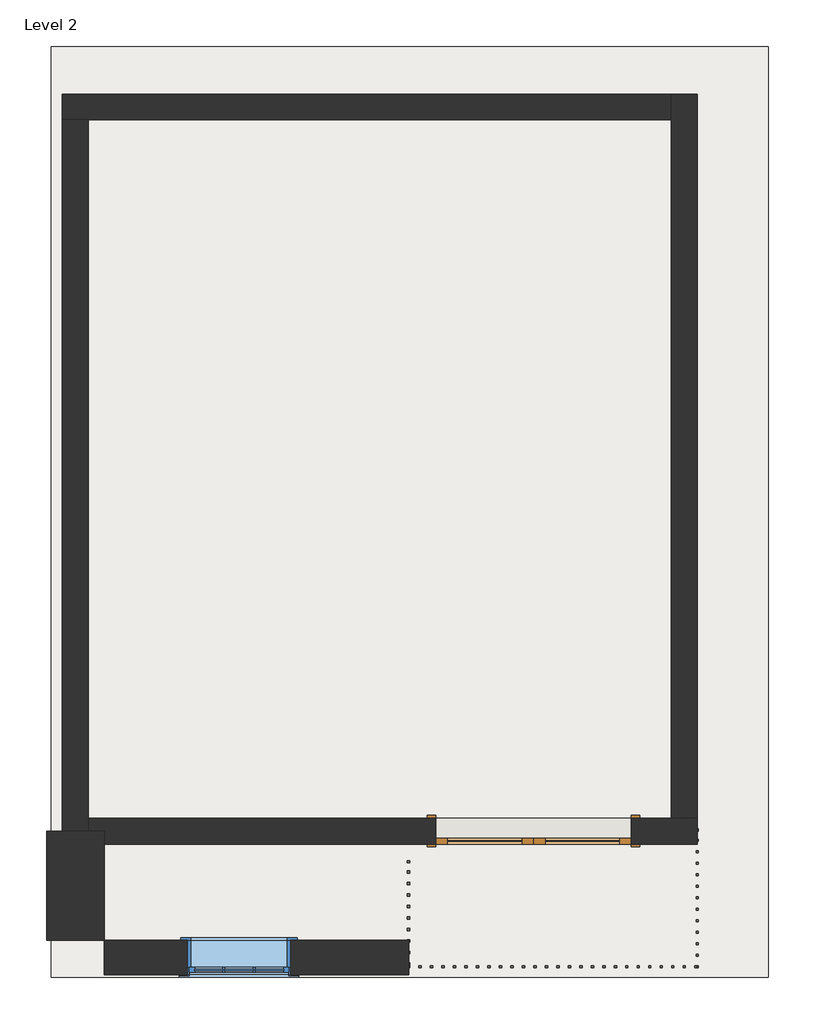
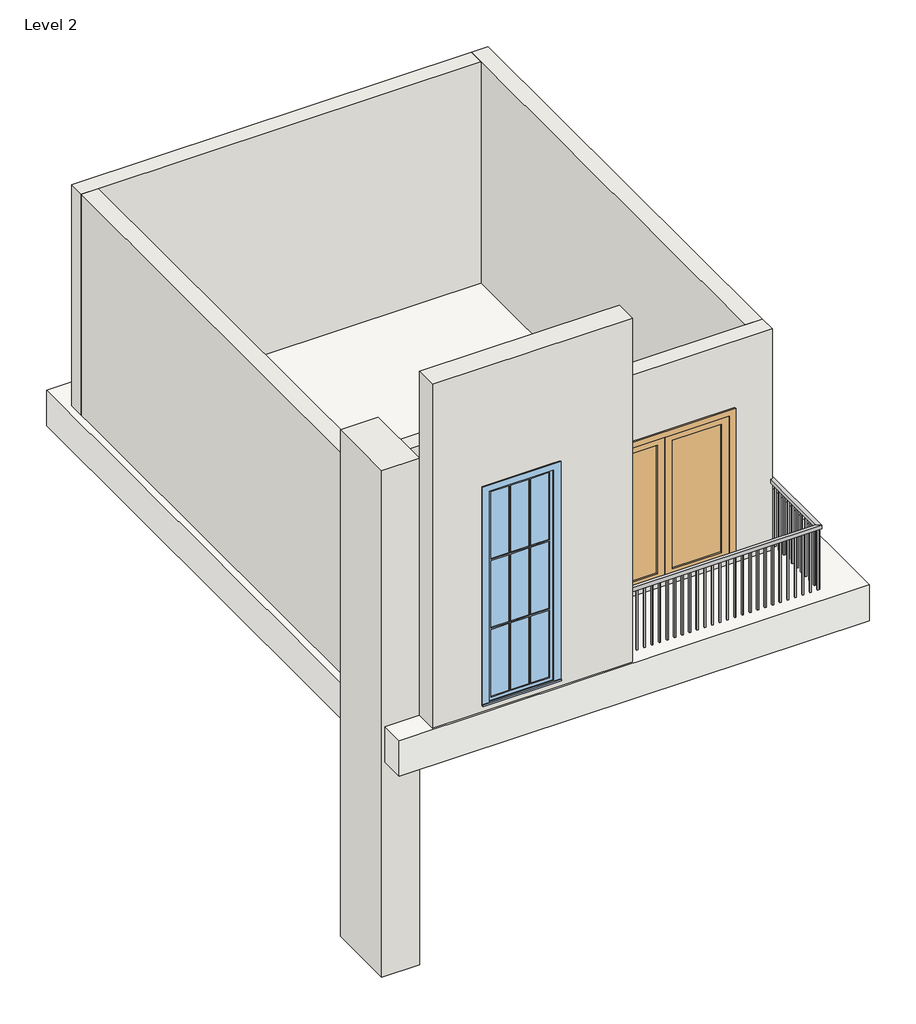
# One storey: 6 walls, 1 door, 1 railing, 1 roof, 1 window.
"""IFC4 building model written with IfcOpenShell, lengths in millimetres."""

from ifc_helpers import new_model, si_unit, frame, origin, place, context, project, spatial, polyline, outline, extrude, faceted_brep, transform, mapped, element, save
from components import door_423d55ee, window_19f256ab

model = new_model("IFC4")

# Units and contexts
model_context = context("Model", 3, world=origin())
ifc_project = project(units=[si_unit("LENGTHUNIT", "METRE", prefix="MILLI")], contexts=[model_context])

# Site, building, storey
site = spatial("IfcSite", under=ifc_project)
building = spatial("IfcBuilding", under=site)
storey = spatial("IfcBuildingStorey", under=building, Name="Level 2", Elevation=3048.0)

# Door
placement = place(None, origin())
door_shape = door_423d55ee(model_context)
element("IfcDoor", 1, ObjectType="Door-Double-Glass : 68\" x 80\"", at=placement, inside=storey, context=model_context, shape_type="MappedRepresentation", body=[
    mapped(door_shape, transform((-9039.9306534, 4280.4110237, 3657.6), x_axis=(-1.0, 0.0, 0.0), y_axis=(0.0, -1.0, 0.0), z_axis=(0.0, 0.0, 1.0))),
])

# Railing
element("IfcRailing", 2, ObjectType="Handrail - Rectangular", at=placement, inside=storey, context=model_context, shape_type="SolidModel", body=[
    faceted_brep([(-10119.4306534, 4017.6797737, 4572.0), (-10119.4306534, 4017.6797737, 4521.2), (-10170.2306534, 4017.6797737, 4521.2), (-10170.2306534, 4017.6797737, 4572.0), (-10119.4306534, 3103.2797737, 4572.0), (-10119.4306534, 3103.2797737, 4521.2), (-10170.2306534, 3052.4797737, 4521.2), (-10170.2306534, 3052.4797737, 4572.0), (-7617.5306534, 3103.2797737, 4572.0), (-7617.5306534, 3103.2797737, 4521.2), (-7566.7306534, 3052.4797737, 4521.2), (-7566.7306534, 3052.4797737, 4572.0), (-7617.5306534, 4297.0797737, 4572.0), (-7566.7306534, 4297.0797737, 4572.0), (-7566.7306534, 4297.0797737, 4521.2), (-7617.5306534, 4297.0797737, 4521.2)], [[[0, 1, 2, 3]], [[1, 0, 4, 5]], [[2, 1, 5, 6]], [[3, 2, 6, 7]], [[0, 3, 7, 4]], [[5, 4, 8, 9]], [[6, 5, 9, 10]], [[7, 6, 10, 11]], [[4, 7, 11, 8]], [[12, 13, 14, 15]], [[9, 8, 12, 15]], [[10, 9, 15, 14]], [[11, 10, 14, 13]], [[8, 11, 13, 12]]]),
    extrude(outline(polyline([(-7582.6056534, 4185.9547737), (-7601.6556534, 4185.9547737), (-7601.6556534, 4205.0047737), (-7582.6056534, 4205.0047737), (-7582.6056534, 4185.9547737)])), frame((0.0, 0.0, 3657.6), z_axis=(0.0, 0.0, 1.0), x_axis=(1.0, 0.0, 0.0)), (0.0, 0.0, 1.0), 863.6),
    extrude(outline(polyline([(-7582.6056534, 4084.3547737), (-7601.6556534, 4084.3547737), (-7601.6556534, 4103.4047737), (-7582.6056534, 4103.4047737), (-7582.6056534, 4084.3547737)])), frame((0.0, 0.0, 3657.6), z_axis=(0.0, 0.0, 1.0), x_axis=(1.0, 0.0, 0.0)), (0.0, 0.0, 1.0), 863.6),
    extrude(outline(polyline([(-7582.6056534, 3982.7547737), (-7601.6556534, 3982.7547737), (-7601.6556534, 4001.8047737), (-7582.6056534, 4001.8047737), (-7582.6056534, 3982.7547737)])), frame((0.0, 0.0, 3657.6), z_axis=(0.0, 0.0, 1.0), x_axis=(1.0, 0.0, 0.0)), (0.0, 0.0, 1.0), 863.6),
    extrude(outline(polyline([(-7582.6056534, 3881.1547737), (-7601.6556534, 3881.1547737), (-7601.6556534, 3900.2047737), (-7582.6056534, 3900.2047737), (-7582.6056534, 3881.1547737)])), frame((0.0, 0.0, 3657.6), z_axis=(0.0, 0.0, 1.0), x_axis=(1.0, 0.0, 0.0)), (0.0, 0.0, 1.0), 863.6),
    extrude(outline(polyline([(-7582.6056534, 3779.5547737), (-7601.6556534, 3779.5547737), (-7601.6556534, 3798.6047737), (-7582.6056534, 3798.6047737), (-7582.6056534, 3779.5547737)])), frame((0.0, 0.0, 3657.6), z_axis=(0.0, 0.0, 1.0), x_axis=(1.0, 0.0, 0.0)), (0.0, 0.0, 1.0), 863.6),
    extrude(outline(polyline([(-7582.6056534, 3677.9547737), (-7601.6556534, 3677.9547737), (-7601.6556534, 3697.0047737), (-7582.6056534, 3697.0047737), (-7582.6056534, 3677.9547737)])), frame((0.0, 0.0, 3657.6), z_axis=(0.0, 0.0, 1.0), x_axis=(1.0, 0.0, 0.0)), (0.0, 0.0, 1.0), 863.6),
    extrude(outline(polyline([(-7582.6056534, 3576.3547737), (-7601.6556534, 3576.3547737), (-7601.6556534, 3595.4047737), (-7582.6056534, 3595.4047737), (-7582.6056534, 3576.3547737)])), frame((0.0, 0.0, 3657.6), z_axis=(0.0, 0.0, 1.0), x_axis=(1.0, 0.0, 0.0)), (0.0, 0.0, 1.0), 863.6),
    extrude(outline(polyline([(-7582.6056534, 3474.7547737), (-7601.6556534, 3474.7547737), (-7601.6556534, 3493.8047737), (-7582.6056534, 3493.8047737), (-7582.6056534, 3474.7547737)])), frame((0.0, 0.0, 3657.6), z_axis=(0.0, 0.0, 1.0), x_axis=(1.0, 0.0, 0.0)), (0.0, 0.0, 1.0), 863.6),
    extrude(outline(polyline([(-7582.6056534, 3373.1547737), (-7601.6556534, 3373.1547737), (-7601.6556534, 3392.2047737), (-7582.6056534, 3392.2047737), (-7582.6056534, 3373.1547737)])), frame((0.0, 0.0, 3657.6), z_axis=(0.0, 0.0, 1.0), x_axis=(1.0, 0.0, 0.0)), (0.0, 0.0, 1.0), 863.6),
    extrude(outline(polyline([(-7582.6056534, 3271.5547737), (-7601.6556534, 3271.5547737), (-7601.6556534, 3290.6047737), (-7582.6056534, 3290.6047737), (-7582.6056534, 3271.5547737)])), frame((0.0, 0.0, 3657.6), z_axis=(0.0, 0.0, 1.0), x_axis=(1.0, 0.0, 0.0)), (0.0, 0.0, 1.0), 863.6),
    extrude(outline(polyline([(-7582.6056534, 3169.9547737), (-7601.6556534, 3169.9547737), (-7601.6556534, 3189.0047737), (-7582.6056534, 3189.0047737), (-7582.6056534, 3169.9547737)])), frame((0.0, 0.0, 3657.6), z_axis=(0.0, 0.0, 1.0), x_axis=(1.0, 0.0, 0.0)), (0.0, 0.0, 1.0), 863.6),
    extrude(outline(polyline([(-7614.3556534, 3068.3547737), (-7614.3556534, 3087.4047737), (-7595.3056534, 3087.4047737), (-7595.3056534, 3068.3547737), (-7614.3556534, 3068.3547737)])), frame((0.0, 0.0, 3657.6), z_axis=(0.0, 0.0, 1.0), x_axis=(1.0, 0.0, 0.0)), (0.0, 0.0, 1.0), 863.6),
    extrude(outline(polyline([(-7715.9556534, 3068.3547737), (-7715.9556534, 3087.4047737), (-7696.9056534, 3087.4047737), (-7696.9056534, 3068.3547737), (-7715.9556534, 3068.3547737)])), frame((0.0, 0.0, 3657.6), z_axis=(0.0, 0.0, 1.0), x_axis=(1.0, 0.0, 0.0)), (0.0, 0.0, 1.0), 863.6),
    extrude(outline(polyline([(-7817.5556534, 3068.3547737), (-7817.5556534, 3087.4047737), (-7798.5056534, 3087.4047737), (-7798.5056534, 3068.3547737), (-7817.5556534, 3068.3547737)])), frame((0.0, 0.0, 3657.6), z_axis=(0.0, 0.0, 1.0), x_axis=(1.0, 0.0, 0.0)), (0.0, 0.0, 1.0), 863.6),
    extrude(outline(polyline([(-7919.1556534, 3068.3547737), (-7919.1556534, 3087.4047737), (-7900.1056534, 3087.4047737), (-7900.1056534, 3068.3547737), (-7919.1556534, 3068.3547737)])), frame((0.0, 0.0, 3657.6), z_axis=(0.0, 0.0, 1.0), x_axis=(1.0, 0.0, 0.0)), (0.0, 0.0, 1.0), 863.6),
    extrude(outline(polyline([(-8020.7556534, 3068.3547737), (-8020.7556534, 3087.4047737), (-8001.7056534, 3087.4047737), (-8001.7056534, 3068.3547737), (-8020.7556534, 3068.3547737)])), frame((0.0, 0.0, 3657.6), z_axis=(0.0, 0.0, 1.0), x_axis=(1.0, 0.0, 0.0)), (0.0, 0.0, 1.0), 863.6),
    extrude(outline(polyline([(-8122.3556534, 3068.3547737), (-8122.3556534, 3087.4047737), (-8103.3056534, 3087.4047737), (-8103.3056534, 3068.3547737), (-8122.3556534, 3068.3547737)])), frame((0.0, 0.0, 3657.6), z_axis=(0.0, 0.0, 1.0), x_axis=(1.0, 0.0, 0.0)), (0.0, 0.0, 1.0), 863.6),
    extrude(outline(polyline([(-8223.9556534, 3068.3547737), (-8223.9556534, 3087.4047737), (-8204.9056534, 3087.4047737), (-8204.9056534, 3068.3547737), (-8223.9556534, 3068.3547737)])), frame((0.0, 0.0, 3657.6), z_axis=(0.0, 0.0, 1.0), x_axis=(1.0, 0.0, 0.0)), (0.0, 0.0, 1.0), 863.6),
    extrude(outline(polyline([(-8325.5556534, 3068.3547737), (-8325.5556534, 3087.4047737), (-8306.5056534, 3087.4047737), (-8306.5056534, 3068.3547737), (-8325.5556534, 3068.3547737)])), frame((0.0, 0.0, 3657.6), z_axis=(0.0, 0.0, 1.0), x_axis=(1.0, 0.0, 0.0)), (0.0, 0.0, 1.0), 863.6),
    extrude(outline(polyline([(-8427.1556534, 3068.3547737), (-8427.1556534, 3087.4047737), (-8408.1056534, 3087.4047737), (-8408.1056534, 3068.3547737), (-8427.1556534, 3068.3547737)])), frame((0.0, 0.0, 3657.6), z_axis=(0.0, 0.0, 1.0), x_axis=(1.0, 0.0, 0.0)), (0.0, 0.0, 1.0), 863.6),
    extrude(outline(polyline([(-8528.7556534, 3068.3547737), (-8528.7556534, 3087.4047737), (-8509.7056534, 3087.4047737), (-8509.7056534, 3068.3547737), (-8528.7556534, 3068.3547737)])), frame((0.0, 0.0, 3657.6), z_axis=(0.0, 0.0, 1.0), x_axis=(1.0, 0.0, 0.0)), (0.0, 0.0, 1.0), 863.6),
    extrude(outline(polyline([(-8630.3556534, 3068.3547737), (-8630.3556534, 3087.4047737), (-8611.3056534, 3087.4047737), (-8611.3056534, 3068.3547737), (-8630.3556534, 3068.3547737)])), frame((0.0, 0.0, 3657.6), z_axis=(0.0, 0.0, 1.0), x_axis=(1.0, 0.0, 0.0)), (0.0, 0.0, 1.0), 863.6),
    extrude(outline(polyline([(-8731.9556534, 3068.3547737), (-8731.9556534, 3087.4047737), (-8712.9056534, 3087.4047737), (-8712.9056534, 3068.3547737), (-8731.9556534, 3068.3547737)])), frame((0.0, 0.0, 3657.6), z_axis=(0.0, 0.0, 1.0), x_axis=(1.0, 0.0, 0.0)), (0.0, 0.0, 1.0), 863.6),
    extrude(outline(polyline([(-8833.5556534, 3068.3547737), (-8833.5556534, 3087.4047737), (-8814.5056534, 3087.4047737), (-8814.5056534, 3068.3547737), (-8833.5556534, 3068.3547737)])), frame((0.0, 0.0, 3657.6), z_axis=(0.0, 0.0, 1.0), x_axis=(1.0, 0.0, 0.0)), (0.0, 0.0, 1.0), 863.6),
    extrude(outline(polyline([(-8935.1556534, 3068.3547737), (-8935.1556534, 3087.4047737), (-8916.1056534, 3087.4047737), (-8916.1056534, 3068.3547737), (-8935.1556534, 3068.3547737)])), frame((0.0, 0.0, 3657.6), z_axis=(0.0, 0.0, 1.0), x_axis=(1.0, 0.0, 0.0)), (0.0, 0.0, 1.0), 863.6),
    extrude(outline(polyline([(-9036.7556534, 3068.3547737), (-9036.7556534, 3087.4047737), (-9017.7056534, 3087.4047737), (-9017.7056534, 3068.3547737), (-9036.7556534, 3068.3547737)])), frame((0.0, 0.0, 3657.6), z_axis=(0.0, 0.0, 1.0), x_axis=(1.0, 0.0, 0.0)), (0.0, 0.0, 1.0), 863.6),
    extrude(outline(polyline([(-9138.3556534, 3068.3547737), (-9138.3556534, 3087.4047737), (-9119.3056534, 3087.4047737), (-9119.3056534, 3068.3547737), (-9138.3556534, 3068.3547737)])), frame((0.0, 0.0, 3657.6), z_axis=(0.0, 0.0, 1.0), x_axis=(1.0, 0.0, 0.0)), (0.0, 0.0, 1.0), 863.6),
    extrude(outline(polyline([(-9239.9556534, 3068.3547737), (-9239.9556534, 3087.4047737), (-9220.9056534, 3087.4047737), (-9220.9056534, 3068.3547737), (-9239.9556534, 3068.3547737)])), frame((0.0, 0.0, 3657.6), z_axis=(0.0, 0.0, 1.0), x_axis=(1.0, 0.0, 0.0)), (0.0, 0.0, 1.0), 863.6),
    extrude(outline(polyline([(-9341.5556534, 3068.3547737), (-9341.5556534, 3087.4047737), (-9322.5056534, 3087.4047737), (-9322.5056534, 3068.3547737), (-9341.5556534, 3068.3547737)])), frame((0.0, 0.0, 3657.6), z_axis=(0.0, 0.0, 1.0), x_axis=(1.0, 0.0, 0.0)), (0.0, 0.0, 1.0), 863.6),
    extrude(outline(polyline([(-9443.1556534, 3068.3547737), (-9443.1556534, 3087.4047737), (-9424.1056534, 3087.4047737), (-9424.1056534, 3068.3547737), (-9443.1556534, 3068.3547737)])), frame((0.0, 0.0, 3657.6), z_axis=(0.0, 0.0, 1.0), x_axis=(1.0, 0.0, 0.0)), (0.0, 0.0, 1.0), 863.6),
    extrude(outline(polyline([(-9544.7556534, 3068.3547737), (-9544.7556534, 3087.4047737), (-9525.7056534, 3087.4047737), (-9525.7056534, 3068.3547737), (-9544.7556534, 3068.3547737)])), frame((0.0, 0.0, 3657.6), z_axis=(0.0, 0.0, 1.0), x_axis=(1.0, 0.0, 0.0)), (0.0, 0.0, 1.0), 863.6),
    extrude(outline(polyline([(-9646.3556534, 3068.3547737), (-9646.3556534, 3087.4047737), (-9627.3056534, 3087.4047737), (-9627.3056534, 3068.3547737), (-9646.3556534, 3068.3547737)])), frame((0.0, 0.0, 3657.6), z_axis=(0.0, 0.0, 1.0), x_axis=(1.0, 0.0, 0.0)), (0.0, 0.0, 1.0), 863.6),
    extrude(outline(polyline([(-9747.9556534, 3068.3547737), (-9747.9556534, 3087.4047737), (-9728.9056534, 3087.4047737), (-9728.9056534, 3068.3547737), (-9747.9556534, 3068.3547737)])), frame((0.0, 0.0, 3657.6), z_axis=(0.0, 0.0, 1.0), x_axis=(1.0, 0.0, 0.0)), (0.0, 0.0, 1.0), 863.6),
    extrude(outline(polyline([(-9849.5556534, 3068.3547737), (-9849.5556534, 3087.4047737), (-9830.5056534, 3087.4047737), (-9830.5056534, 3068.3547737), (-9849.5556534, 3068.3547737)])), frame((0.0, 0.0, 3657.6), z_axis=(0.0, 0.0, 1.0), x_axis=(1.0, 0.0, 0.0)), (0.0, 0.0, 1.0), 863.6),
    extrude(outline(polyline([(-9951.1556534, 3068.3547737), (-9951.1556534, 3087.4047737), (-9932.1056534, 3087.4047737), (-9932.1056534, 3068.3547737), (-9951.1556534, 3068.3547737)])), frame((0.0, 0.0, 3657.6), z_axis=(0.0, 0.0, 1.0), x_axis=(1.0, 0.0, 0.0)), (0.0, 0.0, 1.0), 863.6),
    extrude(outline(polyline([(-10052.7556534, 3068.3547737), (-10052.7556534, 3087.4047737), (-10033.7056534, 3087.4047737), (-10033.7056534, 3068.3547737), (-10052.7556534, 3068.3547737)])), frame((0.0, 0.0, 3657.6), z_axis=(0.0, 0.0, 1.0), x_axis=(1.0, 0.0, 0.0)), (0.0, 0.0, 1.0), 863.6),
    extrude(outline(polyline([(-10154.3556534, 3112.8047737), (-10135.3056534, 3112.8047737), (-10135.3056534, 3093.7547737), (-10154.3556534, 3093.7547737), (-10154.3556534, 3112.8047737)])), frame((0.0, 0.0, 3657.6), z_axis=(0.0, 0.0, 1.0), x_axis=(1.0, 0.0, 0.0)), (0.0, 0.0, 1.0), 863.6),
    extrude(outline(polyline([(-10154.3556534, 3214.4047737), (-10135.3056534, 3214.4047737), (-10135.3056534, 3195.3547737), (-10154.3556534, 3195.3547737), (-10154.3556534, 3214.4047737)])), frame((0.0, 0.0, 3657.6), z_axis=(0.0, 0.0, 1.0), x_axis=(1.0, 0.0, 0.0)), (0.0, 0.0, 1.0), 863.6),
    extrude(outline(polyline([(-10154.3556534, 3316.0047737), (-10135.3056534, 3316.0047737), (-10135.3056534, 3296.9547737), (-10154.3556534, 3296.9547737), (-10154.3556534, 3316.0047737)])), frame((0.0, 0.0, 3657.6), z_axis=(0.0, 0.0, 1.0), x_axis=(1.0, 0.0, 0.0)), (0.0, 0.0, 1.0), 863.6),
    extrude(outline(polyline([(-10154.3556534, 3417.6047737), (-10135.3056534, 3417.6047737), (-10135.3056534, 3398.5547737), (-10154.3556534, 3398.5547737), (-10154.3556534, 3417.6047737)])), frame((0.0, 0.0, 3657.6), z_axis=(0.0, 0.0, 1.0), x_axis=(1.0, 0.0, 0.0)), (0.0, 0.0, 1.0), 863.6),
    extrude(outline(polyline([(-10154.3556534, 3519.2047737), (-10135.3056534, 3519.2047737), (-10135.3056534, 3500.1547737), (-10154.3556534, 3500.1547737), (-10154.3556534, 3519.2047737)])), frame((0.0, 0.0, 3657.6), z_axis=(0.0, 0.0, 1.0), x_axis=(1.0, 0.0, 0.0)), (0.0, 0.0, 1.0), 863.6),
    extrude(outline(polyline([(-10154.3556534, 3620.8047737), (-10135.3056534, 3620.8047737), (-10135.3056534, 3601.7547737), (-10154.3556534, 3601.7547737), (-10154.3556534, 3620.8047737)])), frame((0.0, 0.0, 3657.6), z_axis=(0.0, 0.0, 1.0), x_axis=(1.0, 0.0, 0.0)), (0.0, 0.0, 1.0), 863.6),
    extrude(outline(polyline([(-10154.3556534, 3722.4047737), (-10135.3056534, 3722.4047737), (-10135.3056534, 3703.3547737), (-10154.3556534, 3703.3547737), (-10154.3556534, 3722.4047737)])), frame((0.0, 0.0, 3657.6), z_axis=(0.0, 0.0, 1.0), x_axis=(1.0, 0.0, 0.0)), (0.0, 0.0, 1.0), 863.6),
    extrude(outline(polyline([(-10154.3556534, 3824.0047737), (-10135.3056534, 3824.0047737), (-10135.3056534, 3804.9547737), (-10154.3556534, 3804.9547737), (-10154.3556534, 3824.0047737)])), frame((0.0, 0.0, 3657.6), z_axis=(0.0, 0.0, 1.0), x_axis=(1.0, 0.0, 0.0)), (0.0, 0.0, 1.0), 863.6),
    extrude(outline(polyline([(-10154.3556534, 3925.6047737), (-10135.3056534, 3925.6047737), (-10135.3056534, 3906.5547737), (-10154.3556534, 3906.5547737), (-10154.3556534, 3925.6047737)])), frame((0.0, 0.0, 3657.6), z_axis=(0.0, 0.0, 1.0), x_axis=(1.0, 0.0, 0.0)), (0.0, 0.0, 1.0), 863.6),
    extrude(outline(polyline([(-7601.6556534, 3068.3547737), (-7601.6556534, 3087.4047737), (-7582.6056534, 3087.4047737), (-7582.6056534, 3068.3547737), (-7601.6556534, 3068.3547737)])), frame((0.0, 0.0, 3657.6), z_axis=(0.0, 0.0, 1.0), x_axis=(1.0, 0.0, 0.0)), (0.0, 0.0, 1.0), 863.6),
    extrude(outline(polyline([(-10154.3556534, 3087.4047737), (-10135.3056534, 3087.4047737), (-10135.3056534, 3068.3547737), (-10154.3556534, 3068.3547737), (-10154.3556534, 3087.4047737)])), frame((0.0, 0.0, 3657.6), z_axis=(0.0, 0.0, 1.0), x_axis=(1.0, 0.0, 0.0)), (0.0, 0.0, 1.0), 863.6),
    extrude(outline(polyline([(-7582.6056534, 4278.0297737), (-7601.6556534, 4278.0297737), (-7601.6556534, 4297.0797737), (-7582.6056534, 4297.0797737), (-7582.6056534, 4278.0297737)])), frame((0.0, 0.0, 3657.6), z_axis=(0.0, 0.0, 1.0), x_axis=(1.0, 0.0, 0.0)), (0.0, 0.0, 1.0), 863.6),
    extrude(outline(polyline([(-10154.3556534, 4017.6797737), (-10135.3056534, 4017.6797737), (-10135.3056534, 3998.6297737), (-10154.3556534, 3998.6297737), (-10154.3556534, 4017.6797737)])), frame((0.0, 0.0, 3657.6), z_axis=(0.0, 0.0, 1.0), x_axis=(1.0, 0.0, 0.0)), (0.0, 0.0, 1.0), 863.6),
])

# Roof
element("IfcRoof", 3, ObjectType="Generic - 18\"", at=placement, inside=storey, context=model_context, shape_type="SweptSolid", body=[
    extrude(outline(polyline([(-13301.4465329, 11213.7598519), (-6964.1465329, 11213.7598519), (-6964.1465329, 2984.1598519), (-13301.4465329, 2984.1598519), (-13301.4465329, 11213.7598519)])), frame((0.0, 0.0, 3048.0), z_axis=(0.0, 0.0, 1.0), x_axis=(1.0, 0.0, 0.0)), (0.0, 0.0, 1.0), 508.0),
])

# Walls
element("IfcWall", 4, ObjectType="Generic - 12\"", at=placement, inside=storey, context=model_context, shape_type="Brep", body=[
    faceted_brep([(-10144.8306534, 3314.3598519, 3048.0), (-12837.2306534, 3314.3598519, 3048.0), (-12837.2306534, 3314.3598519, 8451.8321088), (-10449.6306534, 3314.3598519, 8451.8321088), (-10144.8306534, 3314.3598519, 8451.8321088), (-12100.6306534, 3314.3598519, 6693.08663), (-12100.6306534, 3314.3598519, 3645.08663), (-11186.2306534, 3314.3598519, 3645.08663), (-11186.2306534, 3314.3598519, 6693.08663), (-10144.8306534, 3009.5598519, 3048.0), (-10144.8306534, 3009.5598519, 8451.8321088), (-12837.2306534, 3009.5598519, 8451.8321088), (-12837.2306534, 3009.5598519, 3048.0), (-12100.6306534, 3009.5598519, 6693.08663), (-11186.2306534, 3009.5598519, 6693.08663), (-11186.2306534, 3009.5598519, 3645.08663), (-12100.6306534, 3009.5598519, 3645.08663)], [[[0, 1, 2, 3, 4], [5, 6, 7, 8]], [[9, 10, 11, 12], [13, 14, 15, 16]], [[6, 5, 13, 16]], [[7, 6, 16, 15]], [[8, 7, 15, 14]], [[5, 8, 14, 13]], [[1, 0, 9, 12]], [[4, 3, 2, 11, 10]], [[2, 1, 12, 11]], [[0, 4, 10, 9]]]),
])
element("IfcWall", 5, ObjectType="Generic - 12\" Masonry", at=placement, inside=storey, context=model_context, shape_type="Brep", body=[
    faceted_brep([(-13345.2306534, 4278.0297737, 7213.6), (-13345.2306534, 4278.0297737, 0.0), (-13345.2306534, 3314.3598519, 0.0), (-13345.2306534, 3314.3598519, 6705.6), (-13345.2306534, 3314.3598519, 7213.6), (-12837.2306534, 4278.0297737, 0.0), (-12837.2306534, 4278.0297737, 3048.0), (-12837.2306534, 4278.0297737, 6705.6), (-12837.2306534, 4278.0297737, 7213.6), (-12837.2306534, 3314.3598519, 7213.6), (-12837.2306534, 3314.3598519, 6705.6), (-12837.2306534, 3314.3598519, 0.0), (-12837.2306534, 4163.7297737, 0.0), (-13205.5306534, 4278.0297737, 0.0), (-12976.9306534, 4278.0297737, 0.0)], [[[0, 1, 2, 3, 4]], [[5, 6, 7, 8, 9, 10, 11, 12]], [[2, 1, 13, 14, 5, 12, 11]], [[0, 4, 9, 8]], [[0, 8, 7, 6, 5, 14, 13, 1]], [[4, 3, 2, 11, 10, 9]]]),
])
element("IfcWall", 6, ObjectType="Generic - 9\"", at=placement, inside=storey, context=model_context, shape_type="Brep", body=[
    faceted_brep([(-13205.5306534, 10564.5297737, 6705.6), (-13205.5306534, 10564.5297737, 3048.0), (-12976.9306534, 10564.5297737, 3048.0), (-7820.7306534, 10564.5297737, 3048.0), (-7820.7306534, 10564.5297737, 6705.6), (-12976.9306534, 10564.5297737, 6705.6), (-13205.5306534, 10793.1297737, 3048.0), (-13205.5306534, 10793.1297737, 6705.6), (-7820.7306534, 10793.1297737, 6705.6), (-7820.7306534, 10793.1297737, 3048.0)], [[[0, 1, 2, 3, 4, 5]], [[6, 7, 8, 9]], [[3, 2, 1, 6, 9]], [[0, 5, 4, 8, 7]], [[0, 7, 6, 1]], [[3, 9, 8, 4]]]),
])
element("IfcWall", 7, ObjectType="Generic - 9\"", at=placement, inside=storey, context=model_context, shape_type="Brep", body=[
    faceted_brep([(-12976.9306534, 4278.0297737, 6705.6), (-12976.9306534, 4278.0297737, 3048.0), (-12976.9306534, 4392.3297737, 3048.0), (-12976.9306534, 10564.5297737, 3048.0), (-12976.9306534, 10564.5297737, 6705.6), (-12976.9306534, 4392.3297737, 6705.6), (-13205.5306534, 4278.0297737, 3048.0), (-13205.5306534, 4278.0297737, 6705.6), (-13205.5306534, 10564.5297737, 6705.6), (-13205.5306534, 10564.5297737, 3048.0)], [[[0, 1, 2, 3, 4, 5]], [[6, 7, 8, 9]], [[3, 2, 1, 6, 9]], [[0, 5, 4, 8, 7]], [[3, 9, 8, 4]], [[0, 7, 6, 1]]]),
])
element("IfcWall", 8, ObjectType="Generic - 9\"", at=placement, inside=storey, context=model_context, shape_type="Brep", body=[
    faceted_brep([(-7592.1306534, 4392.3297737, 6705.6), (-7592.1306534, 4392.3297737, 3048.0), (-7820.7306534, 4392.3297737, 3048.0), (-12976.9306534, 4392.3297737, 3048.0), (-12976.9306534, 4392.3297737, 6705.6), (-7820.7306534, 4392.3297737, 6705.6), (-8176.3306534, 4392.3297737, 3657.6), (-8176.3306534, 4392.3297737, 5689.6), (-9903.5306534, 4392.3297737, 5689.6), (-9903.5306534, 4392.3297737, 3657.6), (-7592.1306534, 4163.7297737, 3048.0), (-7592.1306534, 4163.7297737, 6705.6), (-12837.2306534, 4163.7297737, 6705.6), (-12837.2306534, 4163.7297737, 3048.0), (-8176.3306534, 4163.7297737, 3657.6), (-9903.5306534, 4163.7297737, 3657.6), (-9903.5306534, 4163.7297737, 5689.6), (-8176.3306534, 4163.7297737, 5689.6), (-12837.2306534, 4278.0297737, 3048.0), (-12976.9306534, 4278.0297737, 3048.0), (-12976.9306534, 4278.0297737, 6705.6), (-12837.2306534, 4278.0297737, 6705.6)], [[[0, 1, 2, 3, 4, 5], [6, 7, 8, 9]], [[10, 11, 12, 13], [14, 15, 16, 17]], [[3, 2, 1, 10, 13, 18, 19]], [[0, 5, 4, 20, 21, 12, 11]], [[0, 11, 10, 1]], [[15, 14, 6, 9]], [[16, 15, 9, 8]], [[17, 16, 8, 7]], [[14, 17, 7, 6]], [[3, 19, 20, 4]], [[20, 19, 18, 21]], [[21, 18, 13, 12]]]),
])
element("IfcWall", 9, ObjectType="Generic - 9\"", at=placement, inside=storey, context=model_context, shape_type="Brep", body=[
    faceted_brep([(-7820.7306534, 10793.1297737, 6705.6), (-7820.7306534, 10793.1297737, 3048.0), (-7820.7306534, 10564.5297737, 3048.0), (-7820.7306534, 4392.3297737, 3048.0), (-7820.7306534, 4392.3297737, 6705.6), (-7820.7306534, 10564.5297737, 6705.6), (-7592.1306534, 10793.1297737, 3048.0), (-7592.1306534, 10793.1297737, 6705.6), (-7592.1306534, 4392.3297737, 6705.6), (-7592.1306534, 4392.3297737, 3048.0)], [[[0, 1, 2, 3, 4, 5]], [[6, 7, 8, 9]], [[3, 2, 1, 6, 9]], [[0, 5, 4, 8, 7]], [[3, 9, 8, 4]], [[0, 7, 6, 1]]]),
])

# Window
window_shape = window_19f256ab(model_context)
element("IfcWindow", 10, ObjectType="Casement 3x3 with Trim : 36\" x 48\"", at=placement, inside=storey, context=model_context, shape_type="MappedRepresentation", body=[
    mapped(window_shape, transform((-11643.4306534, 3161.9598519, 2730.68663), x_axis=(-1.0, 0.0, 0.0), y_axis=(0.0, -1.0, 0.0), z_axis=(0.0, 0.0, 1.0))),
])

save(model, "model.ifc")

# Revit data of these elements
# Type "Door-Double-Glass : 68\" x 80\""
#   Type Mark = "8"
#   Construction Type Id = "opn-d45"
#   Assembly Code = "C1020"
#   Analytic Construction = "Wood frame, double glass door "
#   W = 2' - 10"
#   Thickness = 0' - 2"
#   Thermal Resistance (R) = 1.8150 (h·ft²·°F)/BTU
#   Swing Angle [instance default] = 90.00°
#   Heat Transfer Coefficient (U) = 0.5510 BTU/(h·ft²·°F)
#   Height = 6' - 8"
#   Bottom Rail = 0' - 4"
#   Top Rail = 0' - 4"
#   Stiles = 0' - 4"
#   Trim Projection = 0' - 1"
#   Trim Width = 0' - 3"
#   Width = 5' - 8"
#   Define Thermal Properties by = 1
#   Glazing = Glass
#   Panel Material = Wood - Birch - Solid Stained Light Low Gloss
#   Trim Material = Paint - Sienna
#   Visual Light Transmittance = 0
#   Solar Heat Gain Coefficient = 0
#   Function = (empty or 0)
#   Wall Closure = (empty or 0)
# Type "Handrail - Rectangular"
#   Assembly Code = "C2010400"
#   built-in parameter 1008612 = 0.0416667 (stored number, unit not read)
#   built-in parameter 1008611 = 0.0416667 (stored number, unit not read)
#   built-in parameter 1008609 = 0.333333 (stored number, unit not read)
#   built-in parameter 1008604 = 0.166667 (stored number, unit not read)
#   built-in parameter 1008603 = 0.166667 (stored number, unit not read)
#   Railing Height = 3' - 0"
#   built-in parameter 1008630 = 2
#   built-in parameter 1008610 = 2
#   built-in parameter 1008618 = Baluster - Square : 3/4"
# Type "Generic - 18\""
#   Assembly Code = "B1020"
#   Layers, outside or top first: 1' - 8" no material (function 1)
# Type "Generic - 12\""
#   Assembly Code = "B2010"
#   Layers, outside or top first: 1' - 0" no material (function 1)
# Type "Generic - 12\" Masonry"
#   Assembly Code = "B2010"
#   Layers, outside or top first: 1' - 8" "Asphalt Shingle" (function 1)
# Type "Generic - 9\""
#   Assembly Code = "B2010"
#   Layers, outside or top first: 0' - 9" no material (function 1)
# Type "Casement 3x3 with Trim : 36\" x 48\""
#   Type Mark = "13"
#   Construction Type Id = "GSP4R"
#   Assembly Code = "B2020100"
#   Analytic Construction = "1/8 in Pilkington single glazing"
#   Visual Light Transmittance = 0.9
#   Solar Heat Gain Coefficient = 0.78
#   Heat Transfer Coefficient (U) = 0.6496 BTU/(h·ft²·°F)
#   Height = 10' - 0"
#   Default Sill Height = 3' - 0"
#   Trim Projection - Ext. = 0' - 0 1/2"
#   Trim Projection - Int. = 0' - 0 3/4"
#   Trim Width - Exterior = 0' - 3 1/2"
#   Trim Width - Interior = 0' - 3 1/2"
#   Width = 3' - 0"
#   Window Inset = 0' - 0 3/4"
#   Define Thermal Properties by = 1
#   Glass Pane Material = Glass
#   Sash Material = Roofing, EPDM Membrane
#   Trim Exterior Material = Roofing, EPDM Membrane
#   Trim Interior Material = Trim
#   Wall Closure = (empty or 0)
# Element 1 (IfcDoor, "Door-Double-Glass : 68\" x 80\"")
#   Swing Angle = 90.00°
#   Phase Created = New Construction
#   Materials on its faces: "Wood - Birch - Solid Stained Light Low Gloss", "Paint - Sienna", "Glass"
# Element 2 (IfcRailing, "Handrail - Rectangular")
#   built-in parameter 1008621 = 2 (stored number, unit not read)
#   Phase Created = New Construction
# Element 3 (IfcRoof, "Generic - 18\"")
#   built-in parameter 1001705 = 11.6667 (stored number, unit not read)
#   built-in parameter 1001710 = 33615
#   Phase Created = New Construction
#   Materials on its faces: "Default Roof", "Gypsum Wall Board"
# Element 4 (IfcWall, "Generic - 12\"")
#   built-in parameter 1001111 = 0' - 0"
#   Top Offset = 0' - 0"
#   Base Offset = 0' - 0"
#   Unconnected Height = 17' - 8.7493"
#   wall height = 17' - 8.7493"
#   Phase Created = New Construction
#   Base Constraint = Level 2
#   Materials on its faces: "Default Wall"
# Element 5 (IfcWall, "Generic - 12\" Masonry")
#   built-in parameter 1001111 = -10' - 0"
#   Top Offset = 0' - 0"
#   Base Offset = -10' - 0"
#   Unconnected Height = 23' - 8"
#   wall height = 23' - 8"
#   Phase Created = New Construction
#   Base Constraint = Level 2
#   Materials on its faces: "Asphalt Shingle", "Gypsum Wall Board"
# Elements 6, 7, 8, 9 (IfcWall, "Generic - 9\"")
#   Top Offset = 0' - 0"
#   Base Offset = 0' - 0"
#   Unconnected Height = 12' - 0"
#   wall height = 12' - 0"
#   Phase Created = New Construction
#   Base Constraint = Level 2
#   Materials on its faces: "Default Wall"
# Element 10 (IfcWindow, "Casement 3x3 with Trim : 36\" x 48\"")
#   Mark = "3"
#   Phase Created = New Construction
#   Materials on its faces: "Roofing, EPDM Membrane", "Glass", "Trim"
# Materials
#   "Glass": class "Glass", colour RGB 0 128 192, transparency 0.75, Description = "Soda Lime Glass", Cost = 0
#   "Wood - Birch - Solid Stained Light Low Gloss": class "Wood", colour RGB 210 159 95, transparency 0, Cost = 0
#   "Paint - Sienna": colour RGB 118 70 51, transparency 0, Cost = 0
#   "Asphalt Shingle": class "Generic", colour RGB 155 155 155, transparency 0, Description = "Asphalt roofing shingle", Cost = 0
#   "Roofing, EPDM Membrane": class "Generic", colour RGB 127 127 127, transparency 0, Description = "EPDM roof membrane", Cost = 0
#   "Trim": class "Wood", colour RGB 224 178 126, transparency 0
#   "Default Roof": colour RGB 88 101 114, transparency 0
#   "Gypsum Wall Board": class "Generic", colour RGB 127 127 127, transparency 0, Description = "Gypsum Wall Board", Cost = 0
#   "Default Wall": colour RGB 128 128 128, transparency 0
